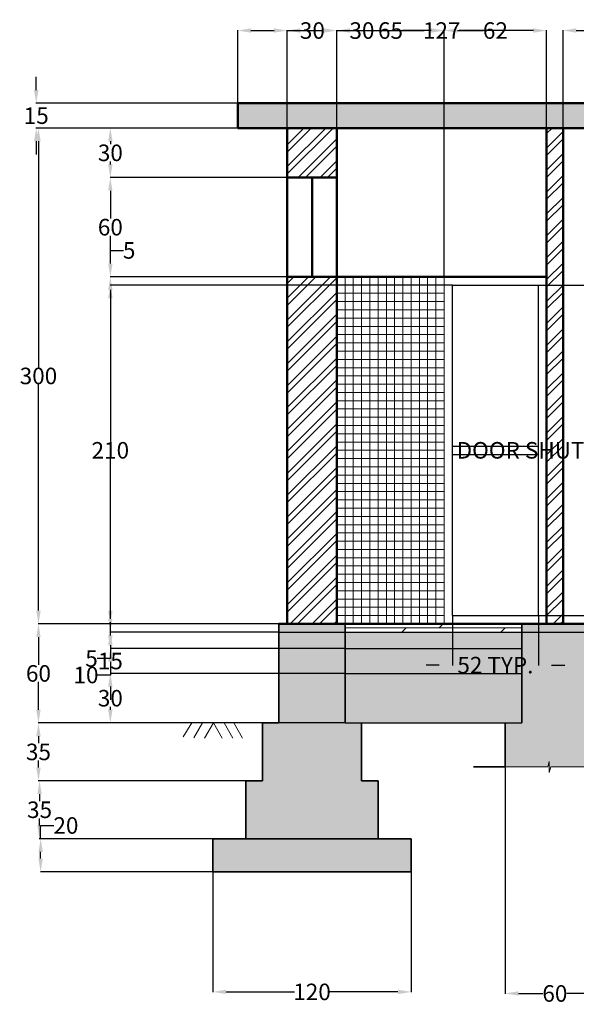
# Model space of a CAD drawing. Units: centimetres. Extents: x 1029 to 1924, y 29 to 653.
# Tile 1 of 2: x 1029 to 1366, y 57 to 653. Entities that reach past the tile are written whole.
import ezdxf

# ---------------------------------------------------------------- set-up
doc = ezdxf.new("R2010")
doc.units = ezdxf.units.CM
doc.header["$MEASUREMENT"] = 0
for name, color, linetype, lineweight in [('A-ANNO-DIMS', 2, 'Continuous', 18), ('A-ANNO-SYMB', 3, 'Continuous', 18), ('A-DETL', 8, 'Continuous', 13), ('A-DOOR', 4, 'Continuous', 25), ('A-FLOR', 3, 'Continuous', 25), ('A-FLOR-PATT', 252, 'Continuous', 13), ('A-WALL', 7, 'Continuous', 50), ('A-WALL-PATT', 8, 'Continuous', 13), ('S-FNDN', 1, 'Continuous', 35), ('S-FNDN-PATT', 8, 'Continuous', 13), ('S-SLAB', 1, 'Continuous', 50)]:
    doc.layers.add(name, color=color, linetype=linetype, lineweight=lineweight)
doc.styles.get("Standard").update_dxf_attribs({"font": 'arial.ttf'})
doc.dimstyles.get("Standard").update_dxf_attribs({"dimtxt": 10, "dimasz": 7.98, "dimexe": 0.18, "dimexo": 0.0625, "dimgap": 0.09, "dimtad": 0, "dimtih": 1, "dimtoh": 1, "dimdec": 0, "dimzin": 0, "dimdsep": 46, "dimtxsty": 'Standard', "dimcen": 0.09, "dimadec": 0, "dimazin": 0, "dimtfac": 1, "dimtdec": 0, "dimtofl": 0, "dimtmove": 0, "dimatfit": 3, "dimfxl": 1, "dimtolj": 1, "dimtzin": 0, "dimarcsym": 0})
pattern_1 = [(50, (-21.744, 120), (14.345204, -1.25504), [1.5, -16.5]), (355, (-21.744, 120), (-2.77503, 15.04384), [1.2, -13.2]), (100.45144, (-20.549, 119.895), (11.57018, 13.7888), [1.2748, -14.02284]), (46.1842, (-21.744, 124), (21.34483, -3.31039), [2.25, -24.75]), (96.6356, (-19.965, 123.724), (18.69324, 19.48237), [1.9122, -21.03428]), (351.1842, (-21.744, 124), (18.69324, 19.48237), [1.8, -19.8]), (21, (-19.744, 123), (11.93814, -8.05238), [1.5, -16.5]), (326, (-19.744, 123), (4.86631, 14.503), [1.2, -13.2]), (71.45144, (-18.749, 122.329), (16.80445, 6.45062), [1.2748, -14.02284]), (37.5, (-21.744, 120), (0.243197, 6.657877), [0, -13.04, 0, -13.4, 0, -13.25]), (7.5, (-21.744, 120), (5.26139, 7.888234), [0, -7.64, 0, -12.74, 0, -5.05]), (327.5, (-26.204, 120), (10.676449, -0.451097), [0, -5, 0, -15.6, 0, -20.7]), (317.5, (-28.204, 120), (11.663723, 2.0021), [0, -6.5, 0, -10.36, 0, -14.7])]

# ---------------------------------------------------------------- blocks, each defined once
blk = doc.blocks.new('*D1')
at = {"layer": 'A-ANNO-DIMS', "color": 0, "lineweight": -2, "transparency": 16777216}
for p, q in [((1039.42, 610.44), (1039.42, 618.42)), ((1161.28, 602.46), (1039.24, 602.46)), ((1161.28, 587.46), (1039.24, 587.46)), ((1039.42, 579.48), (1039.42, 571.5))]:
    blk.add_line(p, q, dxfattribs=at)
at = {"layer": 'A-ANNO-DIMS', "color": 0, "transparency": 16777216}
for points in [[(1038.09, 610.44), (1040.75, 610.44), (1039.42, 602.46)], [(1038.09, 579.48), (1040.75, 579.48), (1039.42, 587.46)]]:
    blk.add_solid(points, dxfattribs=at)
at = {"layer": 'Defpoints', "color": 0, "transparency": 16777216}
for p in [(1161.35, 602.46), (1039.42, 587.46), (1161.35, 587.46)]:
    blk.add_point(p, dxfattribs=at)
at = {"layer": 'A-ANNO-DIMS', "color": 0, "transparency": 16777216, "insert": (1039.42, 594.96), "char_height": 10, "attachment_point": 5}
blk.add_mtext('\\A1;15', dxfattribs=at)
blk = doc.blocks.new('*D2')
at = {"layer": 'A-ANNO-DIMS', "color": 0, "lineweight": -2, "transparency": 16777216}
for p, q in [((1191.28, 587.46), (1040.57, 587.46)), ((1040.75, 579.48), (1040.75, 442.66)), ((1040.75, 295.44), (1040.75, 432.26)), ((1191.28, 287.46), (1040.57, 287.46))]:
    blk.add_line(p, q, dxfattribs=at)
at = {"layer": 'A-ANNO-DIMS', "color": 0, "transparency": 16777216}
for points in [[(1039.42, 579.48), (1042.08, 579.48), (1040.75, 587.46)], [(1039.42, 295.44), (1042.08, 295.44), (1040.75, 287.46)]]:
    blk.add_solid(points, dxfattribs=at)
at = {"layer": 'Defpoints', "color": 0, "transparency": 16777216}
for p in [(1191.35, 587.46), (1040.75, 287.46), (1191.35, 287.46)]:
    blk.add_point(p, dxfattribs=at)
at = {"layer": 'A-ANNO-DIMS', "color": 0, "transparency": 16777216, "insert": (1040.75, 437.46), "char_height": 10, "attachment_point": 5}
blk.add_mtext('\\A1;300', dxfattribs=at)
blk = doc.blocks.new('*D3')
at = {"layer": 'A-ANNO-DIMS', "color": 0, "lineweight": -2, "transparency": 16777216}
for p, q in [((1186.28, 287.46), (1040.57, 287.46)), ((1040.75, 279.48), (1040.75, 262.66)), ((1040.75, 235.44), (1040.75, 252.27)), ((1186.28, 227.46), (1040.57, 227.46))]:
    blk.add_line(p, q, dxfattribs=at)
at = {"layer": 'A-ANNO-DIMS', "color": 0, "transparency": 16777216}
for points in [[(1039.42, 279.48), (1042.08, 279.48), (1040.75, 287.46)], [(1039.42, 235.44), (1042.08, 235.44), (1040.75, 227.46)]]:
    blk.add_solid(points, dxfattribs=at)
at = {"layer": 'Defpoints', "color": 0, "transparency": 16777216}
for p in [(1040.75, 287.46), (1186.35, 287.46), (1186.35, 227.46)]:
    blk.add_point(p, dxfattribs=at)
at = {"layer": 'A-ANNO-DIMS', "color": 0, "transparency": 16777216, "insert": (1040.75, 257.46), "char_height": 10, "attachment_point": 5}
blk.add_mtext('\\A1;60', dxfattribs=at)
blk = doc.blocks.new('*D4')
at = {"layer": 'A-ANNO-DIMS', "color": 0, "lineweight": -2, "transparency": 16777216}
for p, q in [((1176.28, 227.46), (1040.57, 227.46)), ((1040.75, 219.48), (1040.75, 215.16)), ((1040.75, 200.44), (1040.75, 204.76)), ((1176.28, 192.46), (1040.57, 192.46))]:
    blk.add_line(p, q, dxfattribs=at)
at = {"layer": 'A-ANNO-DIMS', "color": 0, "transparency": 16777216}
for points in [[(1039.42, 219.48), (1042.08, 219.48), (1040.75, 227.46)], [(1039.42, 200.44), (1042.08, 200.44), (1040.75, 192.46)]]:
    blk.add_solid(points, dxfattribs=at)
at = {"layer": 'Defpoints', "color": 0, "transparency": 16777216}
for p in [(1040.75, 227.46), (1176.35, 227.46), (1176.35, 192.46)]:
    blk.add_point(p, dxfattribs=at)
at = {"layer": 'A-ANNO-DIMS', "color": 0, "transparency": 16777216, "insert": (1040.75, 209.96), "char_height": 10, "attachment_point": 5}
blk.add_mtext('\\A1;35', dxfattribs=at)
blk = doc.blocks.new('*D5')
at = {"layer": 'A-ANNO-DIMS', "color": 0, "lineweight": -2, "transparency": 16777216}
for p, q in [((1166.28, 192.46), (1041.24, 192.46)), ((1041.42, 184.48), (1041.42, 180.16)), ((1041.42, 165.44), (1041.42, 169.76)), ((1166.28, 157.46), (1041.24, 157.46))]:
    blk.add_line(p, q, dxfattribs=at)
at = {"layer": 'A-ANNO-DIMS', "color": 0, "transparency": 16777216}
for points in [[(1040.09, 184.48), (1042.75, 184.48), (1041.42, 192.46)], [(1040.09, 165.44), (1042.75, 165.44), (1041.42, 157.46)]]:
    blk.add_solid(points, dxfattribs=at)
at = {"layer": 'Defpoints', "color": 0, "transparency": 16777216}
for p in [(1041.42, 192.46), (1166.35, 192.46), (1166.35, 157.46)]:
    blk.add_point(p, dxfattribs=at)
at = {"layer": 'A-ANNO-DIMS', "color": 0, "transparency": 16777216, "insert": (1041.42, 174.96), "char_height": 10, "attachment_point": 5}
blk.add_mtext('\\A1;35', dxfattribs=at)
blk = doc.blocks.new('*D6')
at = {"layer": 'A-ANNO-DIMS', "color": 0, "lineweight": -2, "transparency": 16777216}
for p, q in [((1042.08, 157.46), (1042.08, 165.44)), ((1042.08, 165.44), (1050.06, 165.44)), ((1146.28, 157.46), (1041.9, 157.46)), ((1042.08, 145.44), (1042.08, 149.48)), ((1146.28, 137.46), (1041.9, 137.46))]:
    blk.add_line(p, q, dxfattribs=at)
at = {"layer": 'A-ANNO-DIMS', "color": 0, "transparency": 16777216}
for points in [[(1040.75, 149.48), (1043.41, 149.48), (1042.08, 157.46)], [(1040.75, 145.44), (1043.41, 145.44), (1042.08, 137.46)]]:
    blk.add_solid(points, dxfattribs=at)
at = {"layer": 'Defpoints', "color": 0, "transparency": 16777216}
for p in [(1042.08, 157.46), (1146.35, 157.46), (1146.35, 137.46)]:
    blk.add_point(p, dxfattribs=at)
at = {"layer": 'A-ANNO-DIMS', "color": 0, "transparency": 16777216, "insert": (1057.38, 165.44), "char_height": 10, "attachment_point": 5}
blk.add_mtext('\\A1;20', dxfattribs=at)
blk = doc.blocks.new('*D7')
at = {"layer": 'A-ANNO-DIMS', "color": 0, "lineweight": -2, "transparency": 16777216}
for p, q in [((1146.35, 137.4), (1146.35, 64.57)), ((1266.35, 137.4), (1266.35, 64.57)), ((1154.33, 64.75), (1195.7, 64.75)), ((1258.37, 64.75), (1217, 64.75))]:
    blk.add_line(p, q, dxfattribs=at)
at = {"layer": 'A-ANNO-DIMS', "color": 0, "transparency": 16777216}
for points in [[(1154.33, 66.08), (1154.33, 63.42), (1146.35, 64.75)], [(1258.37, 66.08), (1258.37, 63.42), (1266.35, 64.75)]]:
    blk.add_solid(points, dxfattribs=at)
at = {"layer": 'Defpoints', "color": 0, "transparency": 16777216}
for p in [(1146.35, 137.46), (1266.35, 137.46), (1146.35, 64.75)]:
    blk.add_point(p, dxfattribs=at)
at = {"layer": 'A-ANNO-DIMS', "color": 0, "transparency": 16777216, "insert": (1206.35, 64.75), "char_height": 10, "attachment_point": 5}
blk.add_mtext('\\A1;120', dxfattribs=at)
blk = doc.blocks.new('DOOR-SHUTTER-520')
for p, q in [((0, 200), (52, 200)), ((0, 97.5), (0, 200)), ((52, 97.5), (52, 200)), ((0, 102.5), (52, 102.5)), ((0, 0), (0, 97.5)), ((0, 97.5), (52, 97.5)), ((52, 0), (52, 97.5)), ((0, 0), (52, 0))]:
    blk.add_line(p, q)
blk = doc.blocks.new('*D16')
at = {"layer": 'A-ANNO-DIMS', "color": 0, "lineweight": -2, "transparency": 16777216}
for p, q in [((1343.41, 492.46), (1373.53, 492.46)), ((1373.35, 484.48), (1373.35, 397.73)), ((1373.35, 300.44), (1373.35, 387.2)), ((1343.41, 292.46), (1373.53, 292.46))]:
    blk.add_line(p, q, dxfattribs=at)
at = {"layer": 'A-ANNO-DIMS', "color": 0, "transparency": 16777216}
for points in [[(1372.02, 484.48), (1374.68, 484.48), (1373.35, 492.46)], [(1372.02, 300.44), (1374.68, 300.44), (1373.35, 292.46)]]:
    blk.add_solid(points, dxfattribs=at)
at = {"layer": 'Defpoints', "color": 0, "transparency": 16777216}
for p in [(1343.35, 492.46), (1373.35, 492.46), (1343.35, 292.46)]:
    blk.add_point(p, dxfattribs=at)
at = {"layer": 'A-ANNO-DIMS', "color": 0, "transparency": 16777216, "insert": (1373.35, 392.46), "char_height": 10, "attachment_point": 5}
blk.add_mtext('\\A1;DOOR SHUTTER 200 TYP.', dxfattribs=at)
blk = doc.blocks.new('*D17')
at = {"layer": 'A-ANNO-DIMS', "color": 0, "lineweight": -2, "transparency": 16777216}
for p, q in [((1291.35, 292.4), (1291.35, 262.28)), ((1343.35, 292.4), (1343.35, 262.28)), ((1283.37, 262.46), (1275.39, 262.46)), ((1351.33, 262.46), (1359.31, 262.46))]:
    blk.add_line(p, q, dxfattribs=at)
at = {"layer": 'A-ANNO-DIMS', "color": 0, "transparency": 16777216}
for points in [[(1283.37, 263.79), (1283.37, 261.13), (1291.35, 262.46)], [(1351.33, 263.79), (1351.33, 261.13), (1343.35, 262.46)]]:
    blk.add_solid(points, dxfattribs=at)
at = {"layer": 'Defpoints', "color": 0, "transparency": 16777216}
for p in [(1291.35, 292.46), (1343.35, 292.46), (1343.35, 262.46)]:
    blk.add_point(p, dxfattribs=at)
at = {"layer": 'A-ANNO-DIMS', "color": 0, "transparency": 16777216, "insert": (1317.35, 262.46), "char_height": 10, "attachment_point": 5}
blk.add_mtext('\\A1;52 TYP.', dxfattribs=at)
blk = doc.blocks.new('*D18')
at = {"layer": 'A-ANNO-DIMS', "color": 0, "lineweight": -2, "transparency": 16777216}
for p, q in [((1161.35, 587.52), (1161.35, 646.64)), ((1169.33, 646.46), (1183.37, 646.46)), ((1191.35, 587.52), (1191.35, 646.64)), ((1191.35, 646.46), (1199.33, 646.46))]:
    blk.add_line(p, q, dxfattribs=at)
at = {"layer": 'A-ANNO-DIMS', "color": 0, "transparency": 16777216}
for points in [[(1169.33, 647.79), (1169.33, 645.13), (1161.35, 646.46)], [(1183.37, 647.79), (1183.37, 645.13), (1191.35, 646.46)]]:
    blk.add_solid(points, dxfattribs=at)
at = {"layer": 'Defpoints', "color": 0, "transparency": 16777216}
for p in [(1191.35, 646.46), (1161.35, 587.46), (1191.35, 587.46)]:
    blk.add_point(p, dxfattribs=at)
at = {"layer": 'A-ANNO-DIMS', "color": 0, "transparency": 16777216, "insert": (1206.56, 646.46), "char_height": 10, "attachment_point": 5}
blk.add_mtext('\\A1;30', dxfattribs=at)
blk = doc.blocks.new('*D19')
at = {"layer": 'A-ANNO-DIMS', "color": 0, "lineweight": -2, "transparency": 16777216}
for p, q in [((1191.35, 587.52), (1191.35, 646.64)), ((1199.33, 646.46), (1213.37, 646.46)), ((1221.35, 587.52), (1221.35, 646.64)), ((1221.35, 646.46), (1229.33, 646.46))]:
    blk.add_line(p, q, dxfattribs=at)
at = {"layer": 'A-ANNO-DIMS', "color": 0, "transparency": 16777216}
for points in [[(1199.33, 647.79), (1199.33, 645.13), (1191.35, 646.46)], [(1213.37, 647.79), (1213.37, 645.13), (1221.35, 646.46)]]:
    blk.add_solid(points, dxfattribs=at)
at = {"layer": 'Defpoints', "color": 0, "transparency": 16777216}
for p in [(1221.35, 646.46), (1191.35, 587.46), (1221.35, 587.46)]:
    blk.add_point(p, dxfattribs=at)
at = {"layer": 'A-ANNO-DIMS', "color": 0, "transparency": 16777216, "insert": (1236.56, 646.46), "char_height": 10, "attachment_point": 5}
blk.add_mtext('\\A1;30', dxfattribs=at)
blk = doc.blocks.new('*D20')
at = {"layer": 'A-ANNO-DIMS', "color": 0, "lineweight": -2, "transparency": 16777216}
for p, q in [((1221.35, 587.52), (1221.35, 646.64)), ((1229.33, 646.46), (1274.18, 646.46)), ((1340.37, 646.46), (1295.51, 646.46)), ((1348.35, 587.52), (1348.35, 646.64))]:
    blk.add_line(p, q, dxfattribs=at)
at = {"layer": 'A-ANNO-DIMS', "color": 0, "transparency": 16777216}
for points in [[(1229.33, 647.79), (1229.33, 645.13), (1221.35, 646.46)], [(1340.37, 647.79), (1340.37, 645.13), (1348.35, 646.46)]]:
    blk.add_solid(points, dxfattribs=at)
at = {"layer": 'Defpoints', "color": 0, "transparency": 16777216}
for p in [(1348.35, 646.46), (1221.35, 587.46), (1348.35, 587.46)]:
    blk.add_point(p, dxfattribs=at)
at = {"layer": 'A-ANNO-DIMS', "color": 0, "transparency": 16777216, "insert": (1284.85, 646.46), "char_height": 10, "attachment_point": 5}
blk.add_mtext('\\A1;127', dxfattribs=at)
blk = doc.blocks.new('*D21')
at = {"layer": 'A-ANNO-DIMS', "color": 0, "lineweight": -2, "transparency": 16777216}
for p, q in [((1340.37, 646.46), (1332.39, 646.46)), ((1348.35, 587.52), (1348.35, 646.64)), ((1358.35, 587.52), (1358.35, 646.64)), ((1366.33, 646.46), (1374.31, 646.46))]:
    blk.add_line(p, q, dxfattribs=at)
at = {"layer": 'A-ANNO-DIMS', "color": 0, "transparency": 16777216}
for points in [[(1340.37, 647.79), (1340.37, 645.13), (1348.35, 646.46)], [(1366.33, 647.79), (1366.33, 645.13), (1358.35, 646.46)]]:
    blk.add_solid(points, dxfattribs=at)
at = {"layer": 'Defpoints', "color": 0, "transparency": 16777216}
for p in [(1358.35, 646.46), (1348.35, 587.46), (1358.35, 587.46)]:
    blk.add_point(p, dxfattribs=at)
at = {"layer": 'A-ANNO-DIMS', "color": 0, "transparency": 16777216, "insert": (1381.07, 646.46), "char_height": 10, "attachment_point": 5}
blk.add_mtext('\\A1;10', dxfattribs=at)
blk = doc.blocks.new('*D22')
at = {"layer": 'A-ANNO-DIMS', "color": 0, "lineweight": -2, "transparency": 16777216}
for p, q in [((1358.35, 287.52), (1358.35, 646.64)), ((1366.33, 646.46), (1401.18, 646.46)), ((1457.37, 646.46), (1422.51, 646.46)), ((1465.35, 287.52), (1465.35, 646.64))]:
    blk.add_line(p, q, dxfattribs=at)
at = {"layer": 'A-ANNO-DIMS', "color": 0, "transparency": 16777216}
for points in [[(1366.33, 647.79), (1366.33, 645.13), (1358.35, 646.46)], [(1457.37, 647.79), (1457.37, 645.13), (1465.35, 646.46)]]:
    blk.add_solid(points, dxfattribs=at)
at = {"layer": 'Defpoints', "color": 0, "transparency": 16777216}
for p in [(1465.35, 646.46), (1358.35, 287.46), (1465.35, 287.46)]:
    blk.add_point(p, dxfattribs=at)
at = {"layer": 'A-ANNO-DIMS', "color": 0, "transparency": 16777216, "insert": (1411.85, 646.46), "char_height": 10, "attachment_point": 5}
blk.add_mtext('\\A1;107', dxfattribs=at)
blk = doc.blocks.new('*D26')
at = {"layer": 'A-ANNO-DIMS', "color": 0, "lineweight": -2, "transparency": 16777216}
for p, q in [((1221.35, 497.52), (1221.35, 646.64)), ((1229.33, 646.46), (1246.53, 646.46)), ((1278.37, 646.46), (1261.16, 646.46)), ((1286.35, 497.52), (1286.35, 646.64))]:
    blk.add_line(p, q, dxfattribs=at)
at = {"layer": 'A-ANNO-DIMS', "color": 0, "transparency": 16777216}
for points in [[(1229.33, 647.79), (1229.33, 645.13), (1221.35, 646.46)], [(1278.37, 647.79), (1278.37, 645.13), (1286.35, 646.46)]]:
    blk.add_solid(points, dxfattribs=at)
at = {"layer": 'Defpoints', "color": 0, "transparency": 16777216}
for p in [(1286.35, 646.46), (1221.35, 497.46), (1286.35, 497.46)]:
    blk.add_point(p, dxfattribs=at)
at = {"layer": 'A-ANNO-DIMS', "color": 0, "transparency": 16777216, "insert": (1253.85, 646.46), "char_height": 10, "attachment_point": 5}
blk.add_mtext('\\A1;65', dxfattribs=at)
blk = doc.blocks.new('*D27')
at = {"layer": 'A-ANNO-DIMS', "color": 0, "lineweight": -2, "transparency": 16777216}
for p, q in [((1286.35, 497.52), (1286.35, 646.64)), ((1294.33, 646.46), (1310.12, 646.46)), ((1340.37, 646.46), (1324.58, 646.46)), ((1348.35, 497.52), (1348.35, 646.64))]:
    blk.add_line(p, q, dxfattribs=at)
at = {"layer": 'A-ANNO-DIMS', "color": 0, "transparency": 16777216}
for points in [[(1294.33, 647.79), (1294.33, 645.13), (1286.35, 646.46)], [(1340.37, 647.79), (1340.37, 645.13), (1348.35, 646.46)]]:
    blk.add_solid(points, dxfattribs=at)
at = {"layer": 'Defpoints', "color": 0, "transparency": 16777216}
for p in [(1348.35, 646.46), (1286.35, 497.46), (1348.35, 497.46)]:
    blk.add_point(p, dxfattribs=at)
at = {"layer": 'A-ANNO-DIMS', "color": 0, "transparency": 16777216, "insert": (1317.35, 646.46), "char_height": 10, "attachment_point": 5}
blk.add_mtext('\\A1;62', dxfattribs=at)
blk = doc.blocks.new('*D35')
at = {"layer": 'A-ANNO-DIMS', "color": 0, "lineweight": -2, "transparency": 16777216}
for p, q in [((1084.27, 505.44), (1084.27, 513.42)), ((1084.27, 513.42), (1092.25, 513.42)), ((1286.28, 497.46), (1084.09, 497.46)), ((1291.28, 492.46), (1084.09, 492.46)), ((1084.27, 484.48), (1084.27, 476.5))]:
    blk.add_line(p, q, dxfattribs=at)
at = {"layer": 'A-ANNO-DIMS', "color": 0, "transparency": 16777216}
for points in [[(1082.94, 505.44), (1085.6, 505.44), (1084.27, 497.46)], [(1082.94, 484.48), (1085.6, 484.48), (1084.27, 492.46)]]:
    blk.add_solid(points, dxfattribs=at)
at = {"layer": 'Defpoints', "color": 0, "transparency": 16777216}
for p in [(1084.27, 497.46), (1286.35, 497.46), (1291.35, 492.46)]:
    blk.add_point(p, dxfattribs=at)
at = {"layer": 'A-ANNO-DIMS', "color": 0, "transparency": 16777216, "insert": (1095.66, 513.42), "char_height": 10, "attachment_point": 5}
blk.add_mtext('\\A1;5', dxfattribs=at)
blk = doc.blocks.new('*D36')
at = {"layer": 'A-ANNO-DIMS', "color": 0, "lineweight": -2, "transparency": 16777216}
for p, q in [((1191.28, 557.46), (1084.09, 557.46)), ((1084.27, 549.48), (1084.27, 532.66)), ((1084.27, 505.44), (1084.27, 522.27)), ((1191.28, 497.46), (1084.09, 497.46))]:
    blk.add_line(p, q, dxfattribs=at)
at = {"layer": 'A-ANNO-DIMS', "color": 0, "transparency": 16777216}
for points in [[(1082.94, 549.48), (1085.6, 549.48), (1084.27, 557.46)], [(1082.94, 505.44), (1085.6, 505.44), (1084.27, 497.46)]]:
    blk.add_solid(points, dxfattribs=at)
at = {"layer": 'Defpoints', "color": 0, "transparency": 16777216}
for p in [(1084.27, 557.46), (1191.35, 557.46), (1191.35, 497.46)]:
    blk.add_point(p, dxfattribs=at)
at = {"layer": 'A-ANNO-DIMS', "color": 0, "transparency": 16777216, "insert": (1084.27, 527.46), "char_height": 10, "attachment_point": 5}
blk.add_mtext('\\A1;60', dxfattribs=at)
blk = doc.blocks.new('*D37')
at = {"layer": 'A-ANNO-DIMS', "color": 0, "lineweight": -2, "transparency": 16777216}
for p, q in [((1191.28, 587.46), (1084.09, 587.46)), ((1084.27, 579.48), (1084.27, 577.66)), ((1084.27, 565.44), (1084.27, 567.26)), ((1191.28, 557.46), (1084.09, 557.46))]:
    blk.add_line(p, q, dxfattribs=at)
at = {"layer": 'A-ANNO-DIMS', "color": 0, "transparency": 16777216}
for points in [[(1082.94, 579.48), (1085.6, 579.48), (1084.27, 587.46)], [(1082.94, 565.44), (1085.6, 565.44), (1084.27, 557.46)]]:
    blk.add_solid(points, dxfattribs=at)
at = {"layer": 'Defpoints', "color": 0, "transparency": 16777216}
for p in [(1084.27, 587.46), (1191.35, 587.46), (1191.35, 557.46)]:
    blk.add_point(p, dxfattribs=at)
at = {"layer": 'A-ANNO-DIMS', "color": 0, "transparency": 16777216, "insert": (1084.27, 572.46), "char_height": 10, "attachment_point": 5}
blk.add_mtext('\\A1;30', dxfattribs=at)
blk = doc.blocks.new('*D38')
at = {"layer": 'A-ANNO-DIMS', "color": 0, "lineweight": -2, "transparency": 16777216}
for p, q in [((1191.28, 497.46), (1084.09, 497.46)), ((1084.27, 489.48), (1084.27, 397.66)), ((1084.27, 295.44), (1084.27, 387.27)), ((1191.28, 287.46), (1084.09, 287.46))]:
    blk.add_line(p, q, dxfattribs=at)
at = {"layer": 'A-ANNO-DIMS', "color": 0, "transparency": 16777216}
for points in [[(1082.94, 489.48), (1085.6, 489.48), (1084.27, 497.46)], [(1082.94, 295.44), (1085.6, 295.44), (1084.27, 287.46)]]:
    blk.add_solid(points, dxfattribs=at)
at = {"layer": 'Defpoints', "color": 0, "transparency": 16777216}
for p in [(1084.27, 497.46), (1191.35, 497.46), (1191.35, 287.46)]:
    blk.add_point(p, dxfattribs=at)
at = {"layer": 'A-ANNO-DIMS', "color": 0, "transparency": 16777216, "insert": (1084.27, 392.46), "char_height": 10, "attachment_point": 5}
blk.add_mtext('\\A1;210', dxfattribs=at)
blk = doc.blocks.new('*D39')
at = {"layer": 'A-ANNO-DIMS', "color": 0, "lineweight": -2, "transparency": 16777216}
for p, q in [((1084.27, 295.44), (1084.27, 303.42)), ((1186.28, 287.46), (1084.09, 287.46)), ((1186.28, 282.46), (1084.09, 282.46)), ((1084.27, 274.48), (1084.27, 266.5)), ((1084.27, 266.5), (1076.29, 266.5))]:
    blk.add_line(p, q, dxfattribs=at)
at = {"layer": 'A-ANNO-DIMS', "color": 0, "transparency": 16777216}
for points in [[(1082.94, 295.44), (1085.6, 295.44), (1084.27, 287.46)], [(1082.94, 274.48), (1085.6, 274.48), (1084.27, 282.46)]]:
    blk.add_solid(points, dxfattribs=at)
at = {"layer": 'Defpoints', "color": 0, "transparency": 16777216}
for p in [(1186.35, 287.46), (1084.27, 282.46), (1186.35, 282.46)]:
    blk.add_point(p, dxfattribs=at)
at = {"layer": 'A-ANNO-DIMS', "color": 0, "transparency": 16777216, "insert": (1072.89, 266.5), "char_height": 10, "attachment_point": 5}
blk.add_mtext('\\A1;5', dxfattribs=at)
blk = doc.blocks.new('*D40')
at = {"layer": 'A-ANNO-DIMS', "color": 0, "lineweight": -2, "transparency": 16777216}
for p, q in [((1084.27, 290.44), (1084.27, 298.42)), ((1186.28, 282.46), (1084.09, 282.46)), ((1226.28, 272.46), (1084.09, 272.46)), ((1084.27, 264.48), (1084.27, 256.5)), ((1084.27, 256.5), (1076.29, 256.5))]:
    blk.add_line(p, q, dxfattribs=at)
at = {"layer": 'A-ANNO-DIMS', "color": 0, "transparency": 16777216}
for points in [[(1082.94, 290.44), (1085.6, 290.44), (1084.27, 282.46)], [(1082.94, 264.48), (1085.6, 264.48), (1084.27, 272.46)]]:
    blk.add_solid(points, dxfattribs=at)
at = {"layer": 'Defpoints', "color": 0, "transparency": 16777216}
for p in [(1186.35, 282.46), (1084.27, 272.46), (1226.35, 272.46)]:
    blk.add_point(p, dxfattribs=at)
at = {"layer": 'A-ANNO-DIMS', "color": 0, "transparency": 16777216, "insert": (1069.53, 256.5), "char_height": 10, "attachment_point": 5}
blk.add_mtext('\\A1;10', dxfattribs=at)
blk = doc.blocks.new('*D41')
at = {"layer": 'A-ANNO-DIMS', "color": 0, "lineweight": -2, "transparency": 16777216}
for p, q in [((1084.270875, 280.441751), (1084.270875, 288.421751)), ((1226.284555, 272.461751), (1084.090875, 272.461751)), ((1226.284555, 257.461751), (1084.090875, 257.461751)), ((1084.270875, 249.481751), (1084.270875, 241.501751))]:
    blk.add_line(p, q, dxfattribs=at)
at = {"layer": 'A-ANNO-DIMS', "color": 0, "transparency": 16777216}
for points in [[(1082.940875, 280.441751), (1085.600875, 280.441751), (1084.270875, 272.461751)], [(1082.940875, 249.481751), (1085.600875, 249.481751), (1084.270875, 257.461751)]]:
    blk.add_solid(points, dxfattribs=at)
at = {"layer": 'Defpoints', "color": 0, "transparency": 16777216}
for p in [(1226.347055, 272.461751), (1084.270875, 257.461751), (1226.347055, 257.461751)]:
    blk.add_point(p, dxfattribs=at)
at = {"layer": 'A-ANNO-DIMS', "color": 0, "transparency": 16777216, "insert": (1084.270875, 264.961751), "char_height": 10, "attachment_point": 5}
blk.add_mtext('\\A1;15', dxfattribs=at)
blk = doc.blocks.new('*D42')
at = {"layer": 'A-ANNO-DIMS', "color": 0, "lineweight": -2, "transparency": 16777216}
for p, q in [((1226.28, 257.46), (1084.09, 257.46)), ((1084.27, 249.48), (1084.27, 247.66)), ((1084.27, 235.44), (1084.27, 237.26)), ((1226.28, 227.46), (1084.09, 227.46))]:
    blk.add_line(p, q, dxfattribs=at)
at = {"layer": 'A-ANNO-DIMS', "color": 0, "transparency": 16777216}
for points in [[(1082.94, 249.48), (1085.6, 249.48), (1084.27, 257.46)], [(1082.94, 235.44), (1085.6, 235.44), (1084.27, 227.46)]]:
    blk.add_solid(points, dxfattribs=at)
at = {"layer": 'Defpoints', "color": 0, "transparency": 16777216}
for p in [(1226.35, 257.46), (1084.27, 227.46), (1226.35, 227.46)]:
    blk.add_point(p, dxfattribs=at)
at = {"layer": 'A-ANNO-DIMS', "color": 0, "transparency": 16777216, "insert": (1084.27, 242.46), "char_height": 10, "attachment_point": 5}
blk.add_mtext('\\A1;30', dxfattribs=at)
blk = doc.blocks.new('*D43')
at = {"layer": 'A-ANNO-DIMS', "color": 0, "lineweight": -2, "transparency": 16777216}
for p, q in [((1323.35, 200.83), (1323.35, 63.62)), ((1383.35, 200.83), (1383.35, 63.62)), ((1331.33, 63.8), (1346.08, 63.8)), ((1375.37, 63.8), (1360.61, 63.8))]:
    blk.add_line(p, q, dxfattribs=at)
at = {"layer": 'A-ANNO-DIMS', "color": 0, "transparency": 16777216}
for points in [[(1331.33, 65.13), (1331.33, 62.47), (1323.35, 63.8)], [(1375.37, 65.13), (1375.37, 62.47), (1383.35, 63.8)]]:
    blk.add_solid(points, dxfattribs=at)
at = {"layer": 'Defpoints', "color": 0, "transparency": 16777216}
for p in [(1323.35, 200.89), (1383.35, 200.89), (1383.35, 63.8)]:
    blk.add_point(p, dxfattribs=at)
at = {"layer": 'A-ANNO-DIMS', "color": 0, "transparency": 16777216, "insert": (1353.35, 63.8), "char_height": 10, "attachment_point": 5}
blk.add_mtext('\\A1;60', dxfattribs=at)

msp = doc.modelspace()

# ---------------------------------------------------------------- hatches: boundary and pattern name
at = {"layer": 'A-FLOR-PATT'}
h = msp.add_hatch(dxfattribs=at)
h.set_pattern_fill('AR-CONC', color=256, scale=2)
h.set_pattern_definition(pattern_1)
h.paths.add_polyline_path([(1186.347, 287.462), (1186.347, 282.462), (1226.347, 282.462), (1226.347, 287.462)])
h.paths.add_polyline_path([(1373.347, 282.462), (1373.347, 287.462), (1333.347, 287.462), (1333.347, 282.462)])
h.paths.add_polyline_path([(1460.347, 287.462), (1460.347, 282.462), (1500.347, 282.462), (1500.347, 287.462)])
h.paths.add_polyline_path([(1766.347, 287.462), (1766.347, 282.462), (1806.347, 282.462), (1806.347, 287.462)])
h = msp.add_hatch(dxfattribs=at)
h.set_pattern_fill('DOLMIT', color=256, scale=20)
h.set_pattern_definition([(0, (-21.744, 120), (0, 5), []), (45, (-21.744, 120), (-10, 10), [7.07107, -14.14214])])
h.paths.add_polyline_path([(1333.347, 282.462), (1333.347, 287.462), (1226.347, 287.462), (1226.347, 282.462)])
h.paths.add_polyline_path([(1460.347, 282.462), (1460.347, 287.462), (1373.347, 287.462), (1373.347, 282.462)])
h.paths.add_polyline_path([(1766.347, 282.462), (1766.347, 287.462), (1500.347, 287.462), (1500.347, 282.462)])
h = msp.add_hatch(dxfattribs=at)
h.set_pattern_fill('ANSI33', color=256, scale=25)
h.set_pattern_definition([(45, (-21.744, 120), (-4.419417, 4.419417), []), (45, (-17.325, 120), (-4.419417, 4.419417), [3.125, -1.5625])])
h.paths.add_polyline_path([(1236.347, 227.462), (1226.347, 227.462), (1226.347, 282.462), (1186.347, 282.462), (1186.347, 227.462), (1176.347, 227.462), (1176.347, 192.462), (1166.347, 192.462), (1166.347, 157.462), (1246.347, 157.462), (1246.347, 192.462), (1236.347, 192.462)])
h.paths.add_polyline_path([(1510.347, 227.462), (1500.347, 227.462), (1500.347, 282.462), (1460.347, 282.462), (1460.347, 227.462), (1450.347, 227.462), (1450.347, 192.462), (1440.347, 192.462), (1440.347, 157.462), (1520.347, 157.462), (1520.347, 192.462), (1510.347, 192.462)])
h.paths.add_polyline_path([(1333.347, 227.462), (1323.347, 227.462), (1323.347, 200.892), (1349.035, 200.892), (1349.886, 204.258), (1349.886, 197.447), (1350.837, 200.892), (1383.347, 200.892), (1383.347, 227.462), (1373.347, 227.462), (1373.347, 282.462), (1333.347, 282.462)])
h.paths.add_polyline_path([(1756.347, 192.462), (1746.347, 192.462), (1746.347, 157.462), (1826.347, 157.462), (1826.347, 192.462), (1816.347, 192.462), (1816.347, 227.462), (1806.347, 227.462), (1806.347, 282.462), (1766.347, 282.462), (1766.347, 227.462), (1756.347, 227.462)])
h = msp.add_hatch(dxfattribs=at)
h.set_pattern_fill('AR-SAND', color=256, scale=5)
h.set_pattern_definition([(37.5, (-21.744, 120), (-0.314967, 9.63412), [0, -7.6, 0, -8.5, 0, -8.125]), (7.5, (-21.744, 120), (8.84888, 14.11073), [0, -4.1, 0, -6.85, 0, -2.625]), (327.5, (-27.894, 120), (15.57071, 0.028295), [0, -2.5, 0, -9, 0, -11.75]), (317.5, (-27.894, 120), (15.03063, 4.38838), [0, -1.25, 0, -5.9, 0, -6.75])])
h.paths.add_polyline_path([(1226.347, 282.462), (1226.347, 272.462), (1333.347, 272.462), (1333.347, 282.462)])
h.paths.add_polyline_path([(1460.347, 272.462), (1460.347, 282.462), (1373.347, 282.462), (1373.347, 272.462)])
h.paths.add_polyline_path([(1766.347, 272.462), (1766.347, 282.462), (1500.347, 282.462), (1500.347, 272.462)])
h = msp.add_hatch(dxfattribs=at)
h.set_pattern_fill('GRAVEL', color=256, scale=20)
h.set_pattern_definition([(228.01279, (-7.3441, 140), (-160, -180), [2.69072, -266.38176]), (184.96974, (-9.14414, 138), (240, 20), [4.61736, -457.1185]), (132.51045, (-13.7441, 137.6), (200, -220), [3.25576, -322.32065]), (267.27369, (-21.5441, 132.6), (20, 400), [4.20476, -416.27116]), (292.833654, (-21.7441, 128.4), (-100, 240), [4.1231, -408.18746]), (357.27369, (-20.1441, 124.6), (-400, 20), [4.20476, -416.27116]), (37.69424, (-15.94414, 124.4), (-260, -200), [5.56058, -550.49697]), (72.25533, (-11.54414, 127.8), (140, 440), [5.24976, -519.72643]), (121.429566, (-9.9441, 132.8), (-160, 260), [4.219, -417.68146]), (175.23636, (-12.1441, 136.4), (220, -20), [4.81664, -236.01525]), (222.397438, (-16.94414, 136.8), (-240, -220), [6.22896, -616.6675]), (138.81407, (-1.7441, 132.4), (-140, 120), [2.12602, -210.4769]), (171.469234, (-3.3441, 133.8), (260, -40), [4.04474, -400.43023]), (225, (-7.344, 134.4), (-2e-15, -20), [2.82842, -25.45585]), (203.19859, (-8.7441, 136.8), (100, 40), [1.52316, -150.7923]), (291.8014, (-10.144, 136.2), (-20, 60), [2.15406, -105.54924]), (30.96376, (-9.344, 134.2), (60, 40), [3.49858, -113.12046]), (161.56505, (-6.344, 136), (40, -20), [2.52982, -60.71573]), (16.38954, (-21.7441, 136.2), (200, 60), [3.544, -350.8569]), (70.34618, (-18.3441, 137.2), (-80, -220), [2.97322, -294.34815]), (293.19859, (-6.3441, 140), (-40, 100), [3.0463, -149.26916]), (343.61046, (-5.1441, 137.2), (-200, 60), [3.544, -350.8569]), (339.44395, (-21.7441, 123.8), (-100, 40), [3.4176, -167.46247]), (294.77514, (-18.5441, 122.6), (-100, 220), [2.86356, -283.49286]), (66.80141, (-6.1441, 120), (40, 100), [3.0463, -149.26916]), (17.354025, (-4.9441, 122.8), (-260, -80), [3.35262, -331.90847]), (69.44395, (-15.9441, 120), (-40, -100), [1.7088, -169.17127]), (101.30993, (-7.344, 120), (-20, 80), [1.0198, -100.9606]), (165.96376, (-7.544, 121), (60, -20), [4.1231, -78.33901]), (186.009006, (-11.5441, 122), (200, 20), [3.821, -378.27846]), (303.69007, (-9.344, 132.4), (-20, 40), [2.88444, -69.22659]), (353.157227, (-7.74414, 130), (340, -40), [5.03588, -498.55125]), (60.9454, (-2.7441, 129.4), (-80, -140), [2.05912, -203.85348]), (90, (-1.744, 131.2), (-20, 20), [1.2, -18.8]), (120.25644, (-11.9441, 122.6), (80, -140), [2.77848, -275.0704]), (48.01279, (-13.3441, 125), (160, 180), [5.38144, -263.69104]), (0, (-9.744, 129), (20, 20), [5.2, -14.8]), (325.30485, (-4.5441, 129), (200, -140), [3.16228, -313.06549]), (254.0546, (-1.9441, 127.2), (-20, -80), [2.91204, -142.69016]), (207.645975, (-2.74414, 124.4), (-380, -200), [4.7413, -469.38948]), (175.42608, (-6.94414, 122.2), (-260, 20), [5.01598, -496.58147])])
h.paths.add_polyline_path([(1226.347, 257.462), (1226.347, 227.462), (1236.347, 227.462), (1333.347, 227.462), (1333.347, 257.462)])
h.paths.add_polyline_path([(1460.347, 227.462), (1460.347, 257.462), (1373.347, 257.462), (1373.347, 227.462)])
h.paths.add_polyline_path([(1756.347, 227.462), (1766.347, 227.462), (1766.347, 257.462), (1500.347, 257.462), (1500.347, 227.462)])
at = {"layer": 'A-WALL-PATT'}
h = msp.add_hatch(dxfattribs=at)
h.set_pattern_fill('AR-CONC', color=256, scale=2)
h.set_pattern_definition(pattern_1)
h.paths.add_polyline_path([(1831.347, 587.462), (1831.347, 602.462), (1161.347, 602.462), (1161.347, 587.462)])
h.paths.add_polyline_path([(1460.347, 257.462), (1460.347, 272.462), (1373.347, 272.462), (1373.347, 257.462)])
h.paths.add_polyline_path([(1333.347, 257.462), (1333.347, 272.462), (1226.347, 272.462), (1226.347, 257.462)])
h.paths.add_polyline_path([(1766.347, 257.462), (1766.347, 272.462), (1500.347, 272.462), (1500.347, 257.462)])
h = msp.add_hatch(dxfattribs=at)
h.set_pattern_fill('ANSI32', color=256, scale=25)
h.set_pattern_definition([(45, (-21.744, 120), (-6.629126, 6.629126), []), (45, (-17.325, 120), (-6.629126, 6.629126), [])])
h.paths.add_polyline_path([(1221.347, 497.462), (1191.347, 497.462), (1191.347, 287.462), (1221.347, 287.462)])
h.paths.add_polyline_path([(1348.347, 287.462), (1358.347, 287.462), (1358.347, 587.462), (1348.347, 587.462)])
h.paths.add_polyline_path([(1495.347, 587.462), (1465.347, 587.462), (1465.347, 287.462), (1495.347, 287.462)])
h.paths.add_polyline_path([(1771.347, 287.462), (1801.347, 287.462), (1801.347, 587.462), (1771.347, 587.462)])
h.paths.add_polyline_path([(1221.347, 587.462), (1191.347, 587.462), (1191.347, 557.462), (1221.347, 557.462)])
at = {"layer": 'S-FNDN-PATT'}
h = msp.add_hatch(dxfattribs=at)
h.set_pattern_fill('AR-CONC', color=256, scale=2)
h.set_pattern_definition(pattern_1)
h.paths.add_polyline_path([(1146.347, 157.462), (1146.347, 137.462), (1266.347, 137.462), (1266.347, 157.462)])
h.paths.add_polyline_path([(1540.347, 137.462), (1540.347, 157.462), (1420.347, 157.462), (1420.347, 137.462)])
h.paths.add_polyline_path([(1846.347, 137.462), (1846.347, 157.462), (1726.347, 157.462), (1726.347, 137.462)])

# ---------------------------------------------------------------- linework, layer by layer
at = {"layer": 'A-ANNO-SYMB'}
for p, q in [((1133.519, 227.462), (1128.271, 219.091)), ((1140.055, 227.462), (1134.906, 218.398)), ((1146.697, 227.462), (1141.347, 218.195)), ((1146.697, 227.462), (1152.048, 218.195)), ((1153.127, 227.462), (1158.477, 218.195)), ((1158.969, 227.462), (1164.319, 218.195)), ((1349.035, 200.892), (1349.886, 204.258)), ((1349.886, 204.258), (1349.886, 197.447)), ((1323.347, 200.892), (1349.035, 200.892)), ((1349.886, 197.447), (1350.837, 200.892)), ((1350.837, 200.892), (1383.347, 200.892))]:
    msp.add_line(p, q, dxfattribs=at)
at = {"layer": 'A-DETL'}
for p, q in [((1226.347, 497.462), (1226.347, 287.462)), ((1231.347, 497.462), (1231.347, 287.462)), ((1236.347, 497.462), (1236.347, 287.462)), ((1241.347, 497.462), (1241.347, 287.462)), ((1246.347, 497.462), (1246.347, 287.462)), ((1251.347, 497.462), (1251.347, 287.462)), ((1256.347, 497.462), (1256.347, 287.462)), ((1261.347, 497.462), (1261.347, 287.462)), ((1266.347, 497.462), (1266.347, 287.462)), ((1271.347, 497.462), (1271.347, 287.462)), ((1276.347, 497.462), (1276.347, 287.462)), ((1281.347, 497.462), (1281.347, 287.462)), ((1286.347, 287.462), (1286.347, 497.462)), ((1221.347, 492.462), (1286.347, 492.462)), ((1221.347, 487.462), (1286.347, 487.462)), ((1221.347, 482.462), (1286.347, 482.462)), ((1221.347, 477.462), (1286.347, 477.462)), ((1221.347, 472.462), (1286.347, 472.462)), ((1221.347, 467.462), (1286.347, 467.462)), ((1221.347, 462.462), (1286.347, 462.462)), ((1221.347, 457.462), (1286.347, 457.462)), ((1221.347, 452.462), (1286.347, 452.462)), ((1221.347, 447.462), (1286.347, 447.462)), ((1221.347, 442.462), (1286.347, 442.462)), ((1221.347, 437.462), (1286.347, 437.462)), ((1221.347, 432.462), (1286.347, 432.462)), ((1221.347, 427.462), (1286.347, 427.462)), ((1221.347, 422.462), (1286.347, 422.462)), ((1221.347, 417.462), (1286.347, 417.462)), ((1221.347, 412.462), (1286.347, 412.462)), ((1221.347, 407.462), (1286.347, 407.462)), ((1221.347, 402.462), (1286.347, 402.462)), ((1221.347, 397.462), (1286.347, 397.462)), ((1221.347, 392.462), (1286.347, 392.462)), ((1221.347, 387.462), (1286.347, 387.462)), ((1221.347, 382.462), (1286.347, 382.462)), ((1221.347, 377.462), (1286.347, 377.462)), ((1221.347, 372.462), (1286.347, 372.462)), ((1221.347, 367.462), (1286.347, 367.462)), ((1221.347, 362.462), (1286.347, 362.462)), ((1221.347, 357.462), (1286.347, 357.462)), ((1221.347, 352.462), (1286.347, 352.462)), ((1221.347, 347.462), (1286.347, 347.462)), ((1221.347, 342.462), (1286.347, 342.462)), ((1221.347, 337.462), (1286.347, 337.462)), ((1221.347, 332.462), (1286.347, 332.462)), ((1221.347, 327.462), (1286.347, 327.462)), ((1221.347, 322.462), (1286.347, 322.462)), ((1221.347, 317.462), (1286.347, 317.462)), ((1221.347, 312.462), (1286.347, 312.462)), ((1221.347, 307.462), (1286.347, 307.462)), ((1221.347, 302.462), (1286.347, 302.462)), ((1221.347, 297.462), (1286.347, 297.462)), ((1221.347, 292.462), (1286.347, 292.462)), ((1221.347, 287.462), (1286.347, 287.462))]:
    msp.add_line(p, q, dxfattribs=at)
at = {"layer": 'A-FLOR'}
for p, q in [((1186.347, 282.462), (1373.347, 282.462)), ((1226.347, 272.462), (1333.347, 272.462)), ((1226.347, 257.462), (1333.347, 257.462)), ((1176.347, 227.462), (1186.347, 227.462)), ((1226.347, 227.462), (1236.347, 227.462)), ((1236.347, 227.462), (1333.347, 227.462))]:
    msp.add_line(p, q, dxfattribs=at)
at = {"layer": 'A-WALL'}
for p, q in [((1191.347, 587.462), (1191.347, 287.462)), ((1221.347, 587.462), (1221.347, 287.462)), ((1348.347, 287.462), (1348.347, 587.462)), ((1358.347, 287.462), (1358.347, 587.462)), ((1191.347, 557.462), (1221.347, 557.462)), ((1206.347, 557.462), (1206.347, 497.462)), ((1191.347, 497.462), (1221.347, 497.462)), ((1221.347, 497.462), (1348.347, 497.462)), ((1186.347, 287.462), (1226.347, 287.462)), ((1226.347, 287.462), (1766.347, 287.462)), ((1333.347, 287.462), (1373.347, 287.462))]:
    msp.add_line(p, q, dxfattribs=at)
at = {"layer": 'S-FNDN'}
for p, q in [((1186.347, 287.462), (1186.347, 227.462)), ((1226.347, 287.462), (1226.347, 227.462)), ((1333.347, 227.462), (1333.347, 287.462)), ((1176.347, 227.462), (1176.347, 192.462)), ((1236.347, 227.462), (1236.347, 192.462)), ((1236.347, 227.462), (1236.347, 192.462)), ((1323.347, 227.462), (1323.347, 200.892)), ((1323.347, 200.892), (1304.043, 200.892)), ((1166.347, 192.462), (1176.347, 192.462)), ((1166.347, 192.462), (1166.347, 157.462)), ((1236.347, 192.462), (1246.347, 192.462)), ((1246.347, 192.462), (1246.347, 157.462)), ((1146.347, 157.462), (1266.347, 157.462)), ((1146.347, 157.462), (1146.347, 137.462)), ((1266.347, 157.462), (1266.347, 137.462)), ((1146.347, 137.462), (1266.347, 137.462))]:
    msp.add_line(p, q, dxfattribs=at)
at = {"layer": 'S-SLAB'}
for p, q in [((1161.347, 587.462), (1161.347, 602.462)), ((1161.347, 602.462), (1831.347, 602.462)), ((1161.347, 587.462), (1831.347, 587.462)), ((1191.347, 587.462), (1221.347, 587.462))]:
    msp.add_line(p, q, dxfattribs=at)

# ---------------------------------------------------------------- block references
at = {"layer": 'A-DOOR'}
msp.add_blockref('DOOR-SHUTTER-520', (1291.347, 292.462), dxfattribs=at)

# ---------------------------------------------------------------- dimensions: what is measured, and where the dimension line sits
at = {"layer": 'A-ANNO-DIMS'}
for base, p1, p2, picture, middle in [((1191.347, 646.462), (1161.347, 587.462), (1191.347, 587.462), '*D18', (1206.559, 646.462)), ((1221.347, 646.462), (1191.347, 587.462), (1221.347, 587.462), '*D19', (1236.559, 646.462)), ((1348.347, 646.462), (1221.347, 587.462), (1348.347, 587.462), '*D20', (1284.847, 646.462)), ((1286.347, 646.462), (1221.347, 497.462), (1286.347, 497.462), '*D26', (1253.847, 646.462)), ((1348.347, 646.462), (1286.347, 497.462), (1348.347, 497.462), '*D27', (1317.347, 646.462)), ((1358.347, 646.462), (1348.347, 587.462), (1358.347, 587.462), '*D21', (1381.072, 646.462)), ((1465.347, 646.462), (1358.347, 287.462), (1465.347, 287.462), '*D22', (1411.847, 646.462)), ((1383.347, 63.803), (1323.347, 200.892), (1383.347, 200.892), '*D43', (1353.347, 63.803))]:
    dim = msp.add_linear_dim(base=base, p1=p1, p2=p2, dimstyle='Standard', override={"dimdec": 0, "dimlfac": 1, "dimrnd": 0, "dimzin": 0, "dimdsep": 46, "dimlunit": 2}, dxfattribs=at)
    dim.commit()
    dim.dimension.update_dxf_attribs({"geometry": picture, "text_midpoint": middle})
for p1, p2, distance, picture, middle in [((1161.347, 602.462), (1161.347, 587.462), -121.926, '*D1', (1039.421, 594.962)), ((1191.347, 587.462), (1191.347, 287.462), -150.596, '*D2', (1040.751, 437.462)), ((1186.347, 227.462), (1186.347, 287.462), 145.596, '*D3', (1040.751, 257.462)), ((1176.347, 192.462), (1176.347, 227.462), 135.596, '*D4', (1040.751, 209.962)), ((1166.347, 157.462), (1166.347, 192.462), 124.931, '*D5', (1041.416, 174.962)), ((1146.347, 137.462), (1146.347, 157.462), 104.266, '*D6', (1057.382, 165.442)), ((1266.347, 137.462), (1146.347, 137.462), 72.711, '*D7', (1206.347, 64.751))]:
    dim = msp.add_aligned_dim(p1=p1, p2=p2, distance=distance, dimstyle='Standard', override={"dimclrd": 0, "dimclre": 0, "dimclrt": 0}, dxfattribs=at)
    dim.commit()
    dim.dimension.update_dxf_attribs({"geometry": picture, "text_midpoint": middle})
for base, p1, p2, picture, middle in [((1084.271, 587.462), (1191.347, 557.462), (1191.347, 587.462), '*D37', (1084.271, 572.462)), ((1084.271, 557.462), (1191.347, 497.462), (1191.347, 557.462), '*D36', (1084.271, 527.462)), ((1084.271, 497.462), (1291.347, 492.462), (1286.347, 497.462), '*D35', (1095.656, 513.422)), ((1084.271, 497.462), (1191.347, 287.462), (1191.347, 497.462), '*D38', (1084.271, 392.462)), ((1084.271, 272.462), (1186.347, 282.462), (1226.347, 272.462), '*D40', (1069.526, 256.502)), ((1084.271, 282.462), (1186.347, 287.462), (1186.347, 282.462), '*D39', (1072.886, 266.502)), ((1084.271, 257.462), (1226.347, 272.462), (1226.347, 257.462), '*D41', (1084.271, 264.962)), ((1084.271, 227.462), (1226.347, 257.462), (1226.347, 227.462), '*D42', (1084.271, 242.462))]:
    dim = msp.add_linear_dim(base=base, p1=p1, p2=p2, angle=90, dimstyle='Standard', override={"dimdec": 0, "dimlfac": 1, "dimrnd": 0, "dimzin": 0, "dimdsep": 46, "dimlunit": 2}, dxfattribs=at)
    dim.commit()
    dim.dimension.update_dxf_attribs({"geometry": picture, "text_midpoint": middle})
dim = msp.add_linear_dim(base=(1373.347, 492.462), p1=(1343.347, 292.462), p2=(1343.347, 492.462), angle=90, text='DOOR SHUTTER <> TYP.', dimstyle='Standard', override={"dimdec": 0, "dimlfac": 1, "dimrnd": 0, "dimzin": 0, "dimdsep": 46, "dimlunit": 2}, dxfattribs=at)
dim.commit()
dim.dimension.update_dxf_attribs({"geometry": '*D16', "text_midpoint": (1373.347, 392.462)})
dim = msp.add_linear_dim(base=(1343.347, 262.462), p1=(1291.347, 292.462), p2=(1343.347, 292.462), text='<> TYP.', dimstyle='Standard', override={"dimdec": 0, "dimlfac": 1, "dimrnd": 0, "dimzin": 0, "dimdsep": 46, "dimlunit": 2}, dxfattribs=at)
dim.commit()
dim.dimension.update_dxf_attribs({"geometry": '*D17', "text_midpoint": (1317.347, 262.462)})

doc.saveas('drawing.dxf')
